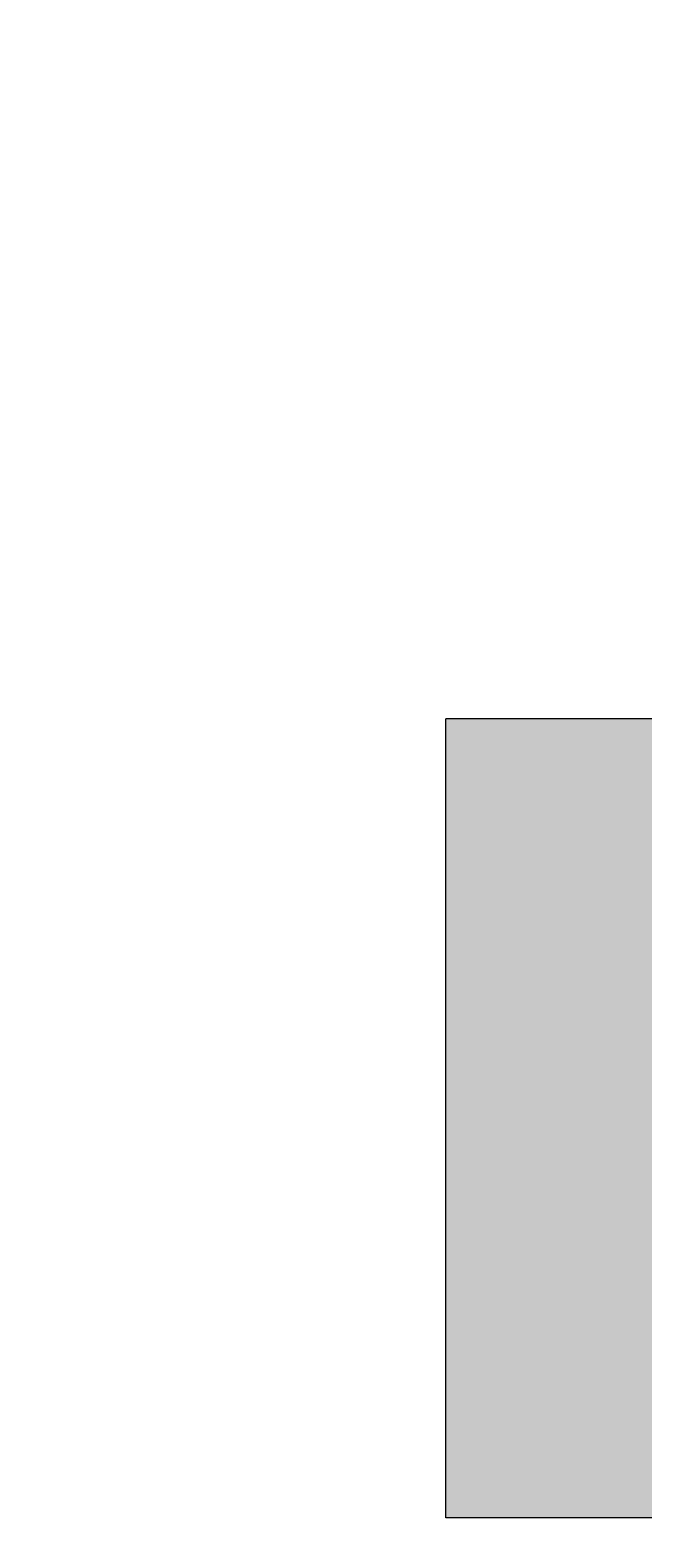
# Model space of a CAD drawing. Units: millimetres. Extents: x 27017497 to 27018854, y 7058029 to 7059154.
# Tile 68 of 91: x 27018355 to 27018367, y 7058144 to 7058174. Entities that reach past the tile are written whole.
import ezdxf

# ---------------------------------------------------------------- set-up
doc = ezdxf.new("R2010")
doc.units = ezdxf.units.MM
for name, color, linetype, lineweight in [('A-ANNO-DIMS', 2, 'Continuous', 18), ('A-FLOR-CASE-PATT', 44, 'Continuous', 13), ('A-FURN', 8, 'Continuous', 18)]:
    doc.layers.add(name, color=color, linetype=linetype, lineweight=lineweight)
doc.layers.add('A-FURN-PATT', color=177, linetype='Continuous', lineweight=13, true_color=0x293189)
doc.styles.get("Standard").update_dxf_attribs({"font": 'arial.ttf'})
doc.dimstyles.get("Standard").update_dxf_attribs({"dimtxt": 0.18, "dimasz": 0.18, "dimexe": 0.18, "dimexo": 0.0625, "dimgap": 0.09, "dimtad": 0, "dimtih": 1, "dimtoh": 1, "dimdec": 4, "dimzin": 0, "dimdsep": 46, "dimtxsty": 'Standard', "dimcen": 0.09, "dimadec": 0, "dimazin": 0, "dimtfac": 1, "dimtdec": 4, "dimtofl": 0, "dimtmove": 0, "dimatfit": 3, "dimfxl": 1, "dimtolj": 1, "dimtzin": 0, "dimarcsym": 0})

# ---------------------------------------------------------------- blocks, each defined once
blk = doc.blocks.new('CAMMAT')
for p, q in [((0.68, -0.07), (1.18, -0.07)), ((1.18, -0.07), (1.18, -0.47)), ((0.68, -0.47), (1.18, -0.47))]:
    blk.add_line(p, q)
blk = doc.blocks.new('*D47')
at = {"layer": 'A-ANNO-DIMS', "color": 0, "lineweight": -2, "transparency": 16777216}
for p, q in [((27017561.166, 7058294.35), (27017561.166, 7058028.6)), ((27018790.606, 7058294.35), (27018790.606, 7058028.6)), ((27017561.346, 7058028.78), (27018175.431, 7058028.78)), ((27018790.426, 7058028.78), (27018176.341, 7058028.78))]:
    blk.add_line(p, q, dxfattribs=at)
at = {"layer": 'A-ANNO-DIMS', "color": 0, "transparency": 16777216}
for points in [[(27017561.346, 7058028.81), (27017561.346, 7058028.75), (27017561.166, 7058028.78)], [(27018790.426, 7058028.81), (27018790.426, 7058028.75), (27018790.606, 7058028.78)]]:
    blk.add_solid(points, dxfattribs=at)
at = {"layer": 'Defpoints', "color": 0, "transparency": 16777216}
for p in [(27017561.166, 7058294.412), (27018790.606, 7058294.412), (27018790.606, 7058028.78)]:
    blk.add_point(p, dxfattribs=at)
at = {"layer": 'A-ANNO-DIMS', "color": 0, "transparency": 16777216, "insert": (27018175.886, 7058028.78), "char_height": 0.18, "attachment_point": 5}
blk.add_mtext('\\A1;1229.4', dxfattribs=at)
blk = doc.blocks.new('*D48')
at = {"layer": 'A-ANNO-DIMS', "color": 0, "lineweight": -2, "transparency": 16777216}
for p, q in [((27018463.498, 7058622.912), (27017497.536, 7058622.912)), ((27017497.716, 7058622.732), (27017497.716, 7058357.753)), ((27017497.716, 7058092.41), (27017497.716, 7058357.389)), ((27018555.129, 7058092.23), (27017497.536, 7058092.23))]:
    blk.add_line(p, q, dxfattribs=at)
at = {"layer": 'A-ANNO-DIMS', "color": 0, "transparency": 16777216}
for points in [[(27017497.686, 7058622.732), (27017497.746, 7058622.732), (27017497.716, 7058622.912)], [(27017497.686, 7058092.41), (27017497.746, 7058092.41), (27017497.716, 7058092.23)]]:
    blk.add_solid(points, dxfattribs=at)
at = {"layer": 'Defpoints', "color": 0, "transparency": 16777216}
for p in [(27018463.561, 7058622.912), (27017497.716, 7058092.23), (27018555.192, 7058092.23)]:
    blk.add_point(p, dxfattribs=at)
at = {"layer": 'A-ANNO-DIMS', "color": 0, "transparency": 16777216, "insert": (27017497.716, 7058357.571), "char_height": 0.18, "attachment_point": 5}
blk.add_mtext('\\A1;530.7', dxfattribs=at)

msp = doc.modelspace()

# ---------------------------------------------------------------- hatches: boundary and pattern name
at = {"layer": 'A-FLOR-CASE-PATT'}
h = msp.add_hatch(color=256, dxfattribs=at)
h.dxf.hatch_style = 1
edge = h.paths.add_edge_path()
edge.add_line((27018341.343, 7058207.055), (27018330.837, 7058207.055))
edge.add_line((27018330.837, 7058207.055), (27018330.837, 7058203.02))
edge.add_line((27018330.837, 7058203.02), (27018338.424, 7058203.02))
edge.add_ellipse((27018338.23, 7058202.551), major_axis=(0.528, 0), ratio=0.888892, start_angle=0, end_angle=90, ccw=False)
edge.add_line((27018338.758, 7058202.551), (27018338.758, 7058202.238))
edge.add_line((27018338.758, 7058202.238), (27018330.837, 7058201.488))
edge.add_line((27018330.837, 7058201.488), (27018330.837, 7058199.747))
edge.add_line((27018330.837, 7058199.747), (27018338.424, 7058199.747))
edge.add_ellipse((27018338.23, 7058199.277), major_axis=(0.528, 0), ratio=0.888892, start_angle=0, end_angle=90, ccw=False)
edge.add_line((27018338.758, 7058199.277), (27018338.758, 7058198.964))
edge.add_line((27018338.758, 7058198.964), (27018330.837, 7058198.215))
edge.add_line((27018330.837, 7058198.215), (27018330.837, 7058193.415))
edge.add_line((27018330.837, 7058193.415), (27018338.284, 7058190.704))
edge.add_ellipse((27018337.942, 7058190.329), major_axis=(0.496, -0.181), ratio=0.888892, start_angle=0, end_angle=90, ccw=False)
edge.add_line((27018338.439, 7058190.148), (27018338.331, 7058189.854))
edge.add_line((27018338.331, 7058189.854), (27018330.837, 7058191.806))
edge.add_line((27018330.837, 7058191.806), (27018330.837, 7058188.22))
edge.add_line((27018330.837, 7058188.22), (27018338.424, 7058188.22))
edge.add_ellipse((27018338.23, 7058187.75), major_axis=(0.528, 0), ratio=0.888892, start_angle=0, end_angle=90, ccw=False)
edge.add_line((27018338.758, 7058187.75), (27018338.758, 7058187.437))
edge.add_line((27018338.758, 7058187.437), (27018330.837, 7058186.688))
edge.add_line((27018330.837, 7058186.688), (27018330.837, 7058181.982))
edge.add_line((27018330.837, 7058181.982), (27018338.424, 7058181.982))
edge.add_ellipse((27018338.23, 7058181.513), major_axis=(0.528, 0), ratio=0.888892, start_angle=0, end_angle=90, ccw=False)
edge.add_line((27018338.758, 7058181.513), (27018338.758, 7058181.199))
edge.add_line((27018338.758, 7058181.199), (27018330.837, 7058180.45))
edge.add_line((27018330.837, 7058180.45), (27018330.837, 7058178.709))
edge.add_line((27018330.837, 7058178.709), (27018338.424, 7058178.709))
edge.add_ellipse((27018338.23, 7058178.239), major_axis=(0.528, 0), ratio=0.888892, start_angle=0, end_angle=90, ccw=False)
edge.add_line((27018338.758, 7058178.239), (27018338.758, 7058177.926))
edge.add_line((27018338.758, 7058177.926), (27018330.837, 7058177.177))
edge.add_line((27018330.837, 7058177.177), (27018330.837, 7058173.878))
edge.add_line((27018330.837, 7058173.878), (27018338.284, 7058171.167))
edge.add_ellipse((27018337.942, 7058170.792), major_axis=(0.496, -0.181), ratio=0.888892, start_angle=0, end_angle=90, ccw=False)
edge.add_line((27018338.439, 7058170.611), (27018338.331, 7058170.317))
edge.add_line((27018338.331, 7058170.317), (27018330.837, 7058172.269))
edge.add_line((27018330.837, 7058172.269), (27018330.837, 7058168.293))
edge.add_line((27018330.837, 7058168.293), (27018338.424, 7058168.293))
edge.add_ellipse((27018338.23, 7058167.824), major_axis=(0.528, 0), ratio=0.888892, start_angle=0, end_angle=90, ccw=False)
edge.add_line((27018338.758, 7058167.824), (27018338.758, 7058167.511))
edge.add_line((27018338.758, 7058167.511), (27018330.837, 7058166.762))
edge.add_line((27018330.837, 7058166.762), (27018330.837, 7058160.389))
edge.add_line((27018330.837, 7058160.389), (27018338.424, 7058160.389))
edge.add_ellipse((27018338.23, 7058159.92), major_axis=(0.528, 0), ratio=0.888892, start_angle=0, end_angle=90, ccw=False)
edge.add_line((27018338.758, 7058159.92), (27018338.758, 7058159.607))
edge.add_line((27018338.758, 7058159.607), (27018330.837, 7058158.858))
edge.add_line((27018330.837, 7058158.858), (27018330.837, 7058157.116))
edge.add_line((27018330.837, 7058157.116), (27018338.424, 7058157.116))
edge.add_ellipse((27018338.23, 7058156.647), major_axis=(0.528, 0), ratio=0.888892, start_angle=0, end_angle=90, ccw=False)
edge.add_line((27018338.758, 7058156.647), (27018338.758, 7058156.334))
edge.add_line((27018338.758, 7058156.334), (27018330.837, 7058155.585))
edge.add_line((27018330.837, 7058155.585), (27018330.837, 7058150.784))
edge.add_line((27018330.837, 7058150.784), (27018338.284, 7058148.073))
edge.add_ellipse((27018337.942, 7058147.698), major_axis=(0.496, -0.181), ratio=0.888892, start_angle=0, end_angle=90, ccw=False)
edge.add_line((27018338.439, 7058147.517), (27018338.331, 7058147.223))
edge.add_line((27018338.331, 7058147.223), (27018330.837, 7058149.175))
edge.add_line((27018330.837, 7058149.175), (27018330.837, 7058145.589))
edge.add_line((27018330.837, 7058145.589), (27018338.424, 7058145.589))
edge.add_ellipse((27018338.23, 7058145.119), major_axis=(0.528, 0), ratio=0.888892, start_angle=0, end_angle=90, ccw=False)
edge.add_line((27018338.758, 7058145.119), (27018338.758, 7058144.806))
edge.add_line((27018338.758, 7058144.806), (27018330.837, 7058144.057))
edge.add_line((27018330.837, 7058144.057), (27018330.837, 7058141.912))
edge.add_line((27018330.837, 7058141.912), (27018341.343, 7058141.912))
edge.add_line((27018341.343, 7058141.912), (27018341.343, 7058207.055))
edge = h.paths.add_edge_path()
edge.add_line((27018330.112, 7058207.055), (27018319.606, 7058207.055))
edge.add_line((27018319.606, 7058207.055), (27018319.606, 7058141.912))
edge.add_line((27018319.606, 7058141.912), (27018330.112, 7058141.912))
edge.add_line((27018330.112, 7058141.912), (27018330.112, 7058144.024))
edge.add_line((27018330.112, 7058144.024), (27018322.543, 7058144.024))
edge.add_ellipse((27018322.736, 7058144.493), major_axis=(0.528, 0), ratio=0.888892, start_angle=180, end_angle=270, ccw=False)
edge.add_line((27018322.208, 7058144.493), (27018322.208, 7058145.291))
edge.add_ellipse((27018322.736, 7058145.119), major_axis=(0.528, 0), ratio=0.888892, start_angle=90, end_angle=180, ccw=False)
edge.add_line((27018322.736, 7058145.589), (27018330.112, 7058145.589))
edge.add_line((27018330.112, 7058145.589), (27018330.112, 7058149.382))
edge.add_line((27018330.112, 7058149.382), (27018322.826, 7058152.034))
edge.add_ellipse((27018323.168, 7058152.409), major_axis=(0.496, -0.181), ratio=0.888892, start_angle=180, end_angle=270, ccw=False)
edge.add_line((27018322.672, 7058152.59), (27018322.945, 7058153.34))
edge.add_ellipse((27018323.382, 7058152.997), major_axis=(0.496, -0.181), ratio=0.888892, start_angle=90, end_angle=180, ccw=False)
edge.add_line((27018323.543, 7058153.439), (27018330.112, 7058151.048))
edge.add_line((27018330.112, 7058151.048), (27018330.112, 7058155.551))
edge.add_line((27018330.112, 7058155.551), (27018322.543, 7058155.551))
edge.add_ellipse((27018322.736, 7058156.021), major_axis=(0.528, 0), ratio=0.888892, start_angle=180, end_angle=270, ccw=False)
edge.add_line((27018322.208, 7058156.021), (27018322.208, 7058156.819))
edge.add_ellipse((27018322.736, 7058156.647), major_axis=(0.528, 0), ratio=0.888892, start_angle=90, end_angle=180, ccw=False)
edge.add_line((27018322.736, 7058157.116), (27018330.112, 7058157.116))
edge.add_line((27018330.112, 7058157.116), (27018330.112, 7058158.824))
edge.add_line((27018330.112, 7058158.824), (27018322.543, 7058158.824))
edge.add_ellipse((27018322.736, 7058159.294), major_axis=(0.528, 0), ratio=0.888892, start_angle=180, end_angle=270, ccw=False)
edge.add_line((27018322.208, 7058159.294), (27018322.208, 7058160.092))
edge.add_ellipse((27018322.736, 7058159.92), major_axis=(0.528, 0), ratio=0.888892, start_angle=90, end_angle=180, ccw=False)
edge.add_line((27018322.736, 7058160.389), (27018330.112, 7058160.389))
edge.add_line((27018330.112, 7058160.389), (27018330.112, 7058166.728))
edge.add_line((27018330.112, 7058166.728), (27018322.543, 7058166.728))
edge.add_ellipse((27018322.736, 7058167.198), major_axis=(0.528, 0), ratio=0.888892, start_angle=180, end_angle=270, ccw=False)
edge.add_line((27018322.208, 7058167.198), (27018322.208, 7058167.996))
edge.add_ellipse((27018322.736, 7058167.824), major_axis=(0.528, 0), ratio=0.888892, start_angle=90, end_angle=180, ccw=False)
edge.add_line((27018322.736, 7058168.293), (27018330.112, 7058168.293))
edge.add_line((27018330.112, 7058168.293), (27018330.112, 7058172.476))
edge.add_line((27018330.112, 7058172.476), (27018322.826, 7058175.128))
edge.add_ellipse((27018323.168, 7058175.503), major_axis=(0.496, -0.181), ratio=0.888892, start_angle=180, end_angle=270, ccw=False)
edge.add_line((27018322.672, 7058175.684), (27018322.945, 7058176.433))
edge.add_ellipse((27018323.382, 7058176.091), major_axis=(0.496, -0.181), ratio=0.888892, start_angle=90, end_angle=180, ccw=False)
edge.add_line((27018323.543, 7058176.533), (27018330.112, 7058174.142))
edge.add_line((27018330.112, 7058174.142), (27018330.112, 7058177.144))
edge.add_line((27018330.112, 7058177.144), (27018322.543, 7058177.144))
edge.add_ellipse((27018322.736, 7058177.613), major_axis=(0.528, 0), ratio=0.888892, start_angle=180, end_angle=270, ccw=False)
edge.add_line((27018322.208, 7058177.613), (27018322.208, 7058178.411))
edge.add_ellipse((27018322.736, 7058178.239), major_axis=(0.528, 0), ratio=0.888892, start_angle=90, end_angle=180, ccw=False)
edge.add_line((27018322.736, 7058178.709), (27018330.112, 7058178.709))
edge.add_line((27018330.112, 7058178.709), (27018330.112, 7058180.417))
edge.add_line((27018330.112, 7058180.417), (27018322.543, 7058180.417))
edge.add_ellipse((27018322.736, 7058180.886), major_axis=(0.528, 0), ratio=0.888892, start_angle=180, end_angle=270, ccw=False)
edge.add_line((27018322.208, 7058180.886), (27018322.208, 7058181.684))
edge.add_ellipse((27018322.736, 7058181.513), major_axis=(0.528, 0), ratio=0.888892, start_angle=90, end_angle=180, ccw=False)
edge.add_line((27018322.736, 7058181.982), (27018330.112, 7058181.982))
edge.add_line((27018330.112, 7058181.982), (27018330.112, 7058186.655))
edge.add_line((27018330.112, 7058186.655), (27018322.543, 7058186.655))
edge.add_ellipse((27018322.736, 7058187.124), major_axis=(0.528, 0), ratio=0.888892, start_angle=180, end_angle=270, ccw=False)
edge.add_line((27018322.208, 7058187.124), (27018322.208, 7058187.922))
edge.add_ellipse((27018322.736, 7058187.75), major_axis=(0.528, 0), ratio=0.888892, start_angle=90, end_angle=180, ccw=False)
edge.add_line((27018322.736, 7058188.22), (27018330.112, 7058188.22))
edge.add_line((27018330.112, 7058188.22), (27018330.112, 7058192.013))
edge.add_line((27018330.112, 7058192.013), (27018322.826, 7058194.665))
edge.add_ellipse((27018323.168, 7058195.04), major_axis=(0.496, -0.181), ratio=0.888892, start_angle=180, end_angle=270, ccw=False)
edge.add_line((27018322.672, 7058195.22), (27018322.945, 7058195.97))
edge.add_ellipse((27018323.382, 7058195.628), major_axis=(0.496, -0.181), ratio=0.888892, start_angle=90, end_angle=180, ccw=False)
edge.add_line((27018323.543, 7058196.069), (27018330.112, 7058193.678))
edge.add_line((27018330.112, 7058193.678), (27018330.112, 7058198.182))
edge.add_line((27018330.112, 7058198.182), (27018322.543, 7058198.182))
edge.add_ellipse((27018322.736, 7058198.651), major_axis=(0.528, 0), ratio=0.888892, start_angle=180, end_angle=270, ccw=False)
edge.add_line((27018322.208, 7058198.651), (27018322.208, 7058199.449))
edge.add_ellipse((27018322.736, 7058199.277), major_axis=(0.528, 0), ratio=0.888892, start_angle=90, end_angle=180, ccw=False)
edge.add_line((27018322.736, 7058199.747), (27018330.112, 7058199.747))
edge.add_line((27018330.112, 7058199.747), (27018330.112, 7058201.455))
edge.add_line((27018330.112, 7058201.455), (27018322.543, 7058201.455))
edge.add_ellipse((27018322.736, 7058201.924), major_axis=(0.528, 0), ratio=0.888892, start_angle=180, end_angle=270, ccw=False)
edge.add_line((27018322.208, 7058201.924), (27018322.208, 7058202.722))
edge.add_ellipse((27018322.736, 7058202.551), major_axis=(0.528, 0), ratio=0.888892, start_angle=90, end_angle=180, ccw=False)
edge.add_line((27018322.736, 7058203.02), (27018330.112, 7058203.02))
edge.add_line((27018330.112, 7058203.02), (27018330.112, 7058207.055))
h.paths.add_polyline_path([(27018341.31, 7058294.412), (27018319.606, 7058294.412), (27018319.606, 7058207.1), (27018341.31, 7058207.1)])
h.paths.add_polyline_path([(27018354.358, 7058255.592), (27018354.358, 7058256.057, -0.414214), (27018354.869, 7058256.569), (27018346.477, 7058256.569, -0.414214), (27018345.197, 7058257.848), (27018345.197, 7058259.128, -0.414214), (27018346.477, 7058260.407), (27018343.868, 7058260.407, 0.290979), (27018341.551, 7058258.934), (27018341.551, 7058242.534, 0.290979), (27018343.868, 7058241.06), (27018346.477, 7058241.06, -0.414214), (27018345.197, 7058242.34), (27018345.197, 7058243.619, -0.414214), (27018346.477, 7058244.899), (27018353.078, 7058244.899, 0.414214), (27018354.358, 7058246.178)])
h.paths.add_polyline_path([(27018356.917, 7058260.407), (27018346.477, 7058260.407, 0.414214), (27018345.197, 7058259.128), (27018345.197, 7058257.848, 0.414214), (27018346.477, 7058256.569), (27018355.637, 7058256.569), (27018355.637, 7058244.899), (27018346.477, 7058244.899, 0.414214), (27018345.197, 7058243.619), (27018345.197, 7058242.34, 0.414214), (27018346.477, 7058241.06), (27018356.917, 7058241.06, 0.414214), (27018359.476, 7058243.619), (27018359.476, 7058257.848, 0.414214)])
h.paths.add_polyline_path([(27018355.637, 7058252.362), (27018355.637, 7058256.057, 0.490314), (27018354.997, 7058256.553, 0.490314), (27018354.358, 7058256.057), (27018354.358, 7058255.592), (27018354.358, 7058245.411, 0.490314), (27018354.997, 7058244.915, 0.490314), (27018355.637, 7058245.411)], flags=17)
at = {"layer": 'A-FURN-PATT'}
h = msp.add_hatch(color=256, dxfattribs=at)
h.dxf.hatch_style = 1
h.paths.add_polyline_path([(27018435.86, 7058218.784, 0.414214), (27018434.267, 7058220.377), (27018385.674, 7058220.377, 0.414214), (27018384.081, 7058218.784), (27018384.081, 7058174.59), (27018387.977, 7058174.891), (27018391.56, 7058175.393), (27018394.078, 7058176.128), (27018395.791, 7058177.21), (27018396.958, 7058178.748), (27018397.838, 7058180.854), (27018398.69, 7058183.639), (27018399.293, 7058180.835), (27018399.836, 7058178.594), (27018400.426, 7058176.691), (27018401.17, 7058174.899), (27018402.177, 7058172.991), (27018403.552, 7058170.741), (27018405.403, 7058167.922), (27018407.838, 7058164.308), (27018410.273, 7058167.922), (27018412.124, 7058170.741), (27018413.499, 7058172.991), (27018414.506, 7058174.899), (27018415.25, 7058176.691), (27018415.84, 7058178.594), (27018416.383, 7058180.835), (27018416.986, 7058183.639), (27018417.838, 7058180.854), (27018418.718, 7058178.748), (27018419.885, 7058177.21), (27018421.598, 7058176.128), (27018424.116, 7058175.393), (27018427.699, 7058174.891), (27018432.604, 7058174.513), (27018435.86, 7058174.329)])
h.paths.add_polyline_path([(27018439.093, 7058174.146), (27018432.604, 7058174.513), (27018427.699, 7058174.891), (27018424.116, 7058175.393), (27018421.598, 7058176.128), (27018419.885, 7058177.21), (27018418.718, 7058178.748), (27018417.838, 7058180.854), (27018416.986, 7058183.639), (27018416.383, 7058180.835), (27018415.84, 7058178.594), (27018415.25, 7058176.691), (27018414.506, 7058174.899), (27018413.499, 7058172.991), (27018412.124, 7058170.741), (27018410.273, 7058167.922), (27018407.838, 7058164.308)])
h.paths.add_polyline_path([(27018403.552, 7058170.741), (27018402.177, 7058172.991), (27018401.17, 7058174.899), (27018400.426, 7058176.691), (27018399.836, 7058178.594), (27018399.293, 7058180.835), (27018398.69, 7058183.639), (27018397.838, 7058180.854), (27018396.958, 7058178.748), (27018395.791, 7058177.21), (27018394.078, 7058176.128), (27018391.56, 7058175.393), (27018387.977, 7058174.891), (27018383.071, 7058174.513), (27018376.583, 7058174.146), (27018407.838, 7058164.308), (27018405.403, 7058167.922)])
h.paths.add_polyline_path([(27018437.469, 7058173.635), (27018407.838, 7058164.308), (27018382.784, 7058172.194), (27018382.784, 7058162.502), (27018437.469, 7058162.502)])
h.paths.add_polyline_path([(27018435.86, 7058162.502), (27018384.081, 7058162.502), (27018384.081, 7058146.294, 0.414214), (27018385.674, 7058144.7), (27018434.267, 7058144.7, 0.414214), (27018435.86, 7058146.294)])
h.paths.add_polyline_path([(27018407.684, 7058159.418, -0.41419), (27018408.879, 7058158.223), (27018408.879, 7058148.664, -0.414237), (27018407.684, 7058147.469), (27018386.224, 7058147.469, -0.41419), (27018385.029, 7058148.663), (27018385.029, 7058158.223, -0.414237), (27018386.224, 7058159.418)], flags=16)
h.paths.add_polyline_path([(27018411.821, 7058159.418), (27018433.28, 7058159.418, -0.41419), (27018434.475, 7058158.223), (27018434.475, 7058148.664, -0.414237), (27018433.28, 7058147.469), (27018411.821, 7058147.469, -0.414214), (27018410.626, 7058148.664), (27018410.626, 7058158.223, -0.414214)], flags=16)
h.paths.add_polyline_path([(27018382.886, 7058160.632), (27018362.971, 7058160.632), (27018362.971, 7058144.7), (27018382.886, 7058144.7)])
h.paths.add_polyline_path([(27018379.136, 7058152.033, -1), (27018367.187, 7058152.033, -1)], flags=16)
h.paths.add_polyline_path([(27018376.861, 7058152.033, -1), (27018369.461, 7058152.033, -1)], flags=0)
h.paths.add_polyline_path([(27018456.97, 7058160.632), (27018437.055, 7058160.632), (27018437.055, 7058144.7), (27018456.97, 7058144.7)])
h.paths.add_polyline_path([(27018453.028, 7058152.033, -1), (27018441.079, 7058152.033, -1)], flags=16)
h.paths.add_polyline_path([(27018450.754, 7058152.033, -1), (27018443.354, 7058152.033, -1)], flags=0)
h.paths.add_polyline_path([(27018434.475, 7058158.223, 0.41419), (27018433.28, 7058159.418), (27018411.821, 7058159.418, 0.414214), (27018410.626, 7058158.223), (27018410.626, 7058148.664, 0.414214), (27018411.821, 7058147.469), (27018433.28, 7058147.469, 0.414237), (27018434.475, 7058148.664)], flags=0)

# ---------------------------------------------------------------- block references
at = {"layer": 'A-FURN', "xscale": 39.82996475819422, "yscale": 39.82996475819422, "zscale": 39.82996475819422, "rotation": 180}
msp.add_blockref('CAMMAT', (27018409.97, 7058141.912), dxfattribs=at)

# ---------------------------------------------------------------- dimensions: what is measured, and where the dimension line sits
at = {"layer": 'A-ANNO-DIMS'}
dim = msp.add_linear_dim(base=(27017497.716, 7058092.23), p1=(27018463.561, 7058622.912), p2=(27018555.192, 7058092.23), angle=90, dimstyle='Standard', override={"dimdec": 1, "dimlfac": 1, "dimrnd": 0, "dimzin": 0, "dimdsep": 46, "dimlunit": 2}, dxfattribs=at)
dim.commit()
dim.dimension.update_dxf_attribs({"geometry": '*D48', "text_midpoint": (27017497.716, 7058357.571)})
dim = msp.add_linear_dim(base=(27018790.606, 7058028.78), p1=(27017561.166, 7058294.412), p2=(27018790.606, 7058294.412), dimstyle='Standard', override={"dimdec": 1, "dimlfac": 1, "dimrnd": 0, "dimzin": 0, "dimdsep": 46, "dimlunit": 2}, dxfattribs=at)
dim.commit()
dim.dimension.update_dxf_attribs({"geometry": '*D47', "text_midpoint": (27018175.886, 7058028.78)})

doc.saveas('drawing.dxf')
